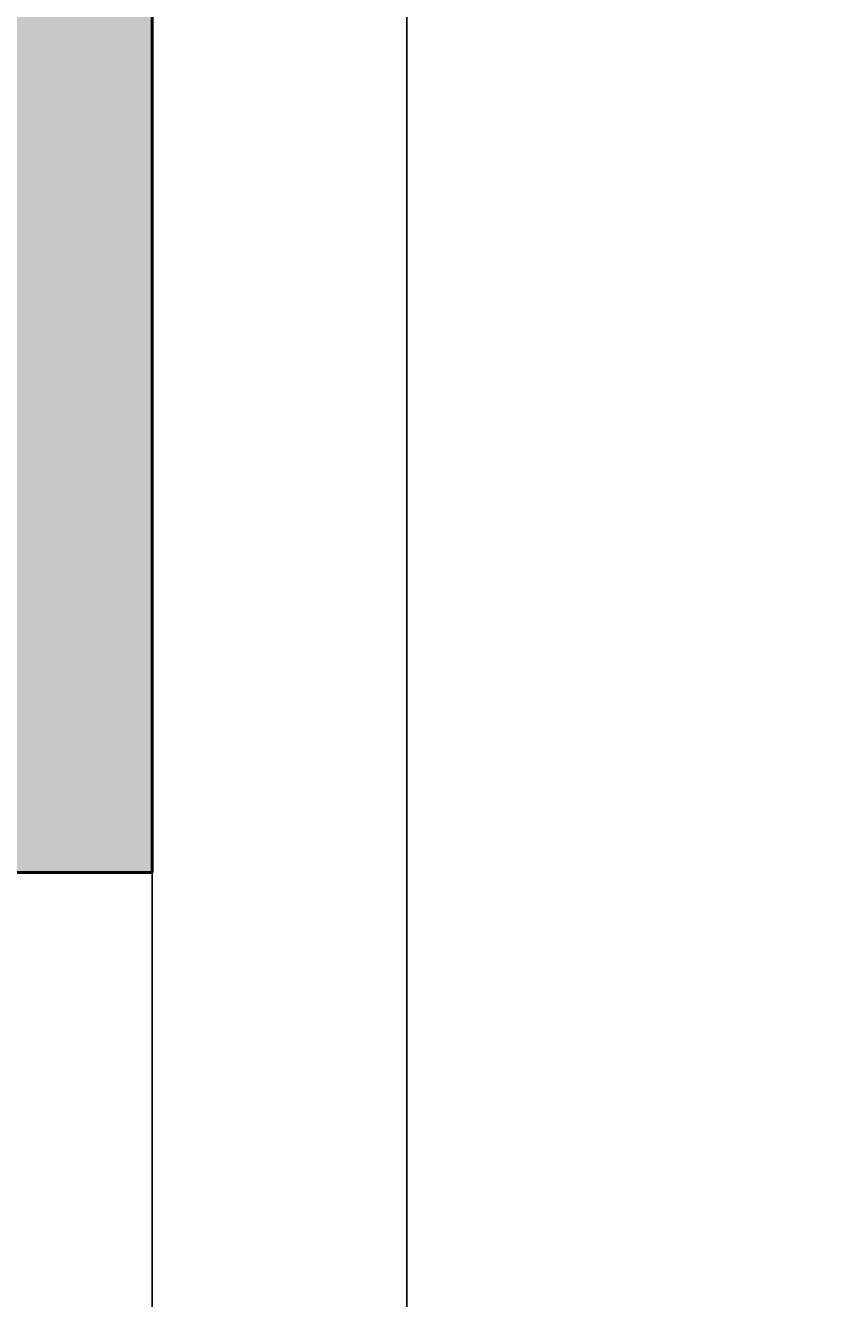
# Model space of a CAD drawing. Units: inches. Extents: x 2307 to 2544, y 2171 to 2540.
# Tile 34 of 52: x 2453 to 2472, y 2377 to 2407. Entities that reach past the tile are written whole.
import ezdxf

# ---------------------------------------------------------------- set-up
doc = ezdxf.new("R2010")
doc.units = ezdxf.units.IN
doc.layers.add('A-ANNO-DIMS', color=2, linetype='Continuous', lineweight=18)
doc.layers.add('A-WALL', color=7, linetype='Continuous', lineweight=50)
doc.layers.add('A-WALL-PATT', color=18, linetype='Continuous', lineweight=13, true_color=0x000000)
doc.styles.get("Standard").update_dxf_attribs({"font": 'arial.ttf'})
doc.dimstyles.get("Standard").update_dxf_attribs({"dimtxt": 0.18, "dimasz": 0.18, "dimexe": 0.18, "dimexo": 0.0625, "dimgap": 0.09, "dimtad": 0, "dimtih": 1, "dimtoh": 1, "dimdec": 4, "dimzin": 0, "dimdsep": 46, "dimtxsty": 'Standard', "dimcen": 0.09, "dimadec": 0, "dimazin": 0, "dimtfac": 1, "dimtdec": 4, "dimtofl": 0, "dimtmove": 0, "dimatfit": 3, "dimfxl": 1, "dimtolj": 1, "dimtzin": 0, "dimarcsym": 0})

# ---------------------------------------------------------------- blocks, each defined once
blk = doc.blocks.new('*D53')
at = {"layer": 'A-ANNO-DIMS', "color": 0, "lineweight": -2, "transparency": 16777216}
for p, q in [((2455.696, 2439.447), (2455.696, 2171.18)), ((2461.696, 2439.447), (2461.696, 2171.18)), ((2455.876, 2171.36), (2458.546, 2171.36)), ((2461.516, 2171.36), (2458.845, 2171.36))]:
    blk.add_line(p, q, dxfattribs=at)
at = {"layer": 'A-ANNO-DIMS', "color": 0, "transparency": 16777216}
for points in [[(2455.876, 2171.39), (2455.876, 2171.33), (2455.696, 2171.36)], [(2461.516, 2171.39), (2461.516, 2171.33), (2461.696, 2171.36)]]:
    blk.add_solid(points, dxfattribs=at)
at = {"layer": 'Defpoints', "color": 0, "transparency": 16777216}
for p in [(2455.696, 2439.51), (2461.696, 2439.51), (2461.696, 2171.36)]:
    blk.add_point(p, dxfattribs=at)
at = {"layer": 'A-ANNO-DIMS', "color": 0, "transparency": 16777216, "insert": (2458.696, 2171.36), "char_height": 0.18, "attachment_point": 5}
blk.add_mtext('\\A1;6', dxfattribs=at)
blk = doc.blocks.new('*D54')
at = {"layer": 'A-ANNO-DIMS', "color": 0, "lineweight": -2, "transparency": 16777216}
for p, q in [((2461.696, 2435.447), (2461.696, 2171.18)), ((2491.696, 2435.447), (2491.696, 2171.18)), ((2461.876, 2171.36), (2476.477, 2171.36)), ((2491.516, 2171.36), (2476.914, 2171.36))]:
    blk.add_line(p, q, dxfattribs=at)
at = {"layer": 'A-ANNO-DIMS', "color": 0, "transparency": 16777216}
for points in [[(2461.876, 2171.39), (2461.876, 2171.33), (2461.696, 2171.36)], [(2491.516, 2171.39), (2491.516, 2171.33), (2491.696, 2171.36)]]:
    blk.add_solid(points, dxfattribs=at)
at = {"layer": 'Defpoints', "color": 0, "transparency": 16777216}
for p in [(2461.696, 2435.51), (2491.696, 2435.51), (2491.696, 2171.36)]:
    blk.add_point(p, dxfattribs=at)
at = {"layer": 'A-ANNO-DIMS', "color": 0, "transparency": 16777216, "insert": (2476.696, 2171.36), "char_height": 0.18, "attachment_point": 5}
blk.add_mtext('\\A1;30', dxfattribs=at)
blk = doc.blocks.new('*D59')
at = {"layer": 'A-ANNO-DIMS', "color": 0, "lineweight": -2, "transparency": 16777216}
for p, q in [((2455.696, 2315.572), (2455.696, 2540.345)), ((2455.876, 2540.165), (2470.477, 2540.165)), ((2485.516, 2540.165), (2470.914, 2540.165)), ((2485.696, 2315.572), (2485.696, 2540.345))]:
    blk.add_line(p, q, dxfattribs=at)
at = {"layer": 'A-ANNO-DIMS', "color": 0, "transparency": 16777216}
for points in [[(2455.876, 2540.195), (2455.876, 2540.135), (2455.696, 2540.165)], [(2485.516, 2540.195), (2485.516, 2540.135), (2485.696, 2540.165)]]:
    blk.add_solid(points, dxfattribs=at)
at = {"layer": 'Defpoints', "color": 0, "transparency": 16777216}
for p in [(2455.696, 2540.165), (2455.696, 2315.51), (2485.696, 2315.51)]:
    blk.add_point(p, dxfattribs=at)
at = {"layer": 'A-ANNO-DIMS', "color": 0, "transparency": 16777216, "insert": (2470.696, 2540.165), "char_height": 0.18, "attachment_point": 5}
blk.add_mtext('\\A1;30', dxfattribs=at)

msp = doc.modelspace()

# ---------------------------------------------------------------- hatches: boundary and pattern name
at = {"layer": 'A-WALL-PATT'}
h = msp.add_hatch(color=256, dxfattribs=at)
h.dxf.hatch_style = 1
h.paths.add_polyline_path([(2433.6935, 2199.5096), (2415.6423, 2199.5096), (2415.6423, 2190.5096), (2433.7832, 2190.5096)], flags=17)
h.paths.add_polyline_path([(2367.6423, 2199.5096), (2335.6958, 2199.5096), (2335.6958, 2307.3983), (2326.6958, 2307.3983), (2326.6958, 2190.5096), (2367.6423, 2190.5096)])
h.paths.add_polyline_path([(2524.6958, 2520.5096), (2496.7832, 2520.5096), (2496.7832, 2515.5149), (2472.7832, 2515.5149), (2472.7832, 2520.5096), (2415.4028, 2520.5096), (2415.4028, 2511.5096), (2451.6958, 2511.5096), (2451.6958, 2439.5096), (2451.6958, 2391.5096), (2445.6958, 2391.5096), (2445.6958, 2387.5096), (2455.6958, 2387.5096), (2455.6958, 2435.5096), (2461.6958, 2435.5096), (2461.6958, 2439.5096), (2455.6958, 2439.5096), (2455.6958, 2511.5096), (2515.6958, 2511.5096), (2515.6958, 2439.5096), (2491.6958, 2439.5096), (2491.6958, 2435.5096), (2515.6958, 2435.5096), (2515.6958, 2319.5096), (2451.6958, 2319.5096), (2451.6958, 2281.5096), (2481.6958, 2281.5096), (2481.6958, 2225.5096), (2485.6958, 2225.5096), (2485.6958, 2285.5096), (2455.6958, 2285.5096), (2455.6958, 2315.5096), (2515.6958, 2315.5096), (2515.6958, 2199.5096), (2469.6952, 2199.5096), (2469.785, 2190.5096), (2524.6958, 2190.5096)])

# ---------------------------------------------------------------- linework, layer by layer
at = {"layer": 'A-WALL'}
for p, q in [((2455.6958, 2387.5096), (2455.6958, 2435.5096)), ((2455.6958, 2435.5096), (2455.6958, 2387.5096)), ((2445.6958, 2387.5096), (2455.6958, 2387.5096))]:
    msp.add_line(p, q, dxfattribs=at)

# ---------------------------------------------------------------- dimensions: what is measured, and where the dimension line sits
at = {"layer": 'A-ANNO-DIMS'}
for base, p1, p2, picture, middle in [((2455.6958, 2540.1649), (2485.6958, 2315.5096), (2455.6958, 2315.5096), '*D59', (2470.6958, 2540.1649)), ((2461.6958, 2171.3596), (2455.6958, 2439.5096), (2461.6958, 2439.5096), '*D53', (2458.6958, 2171.3596)), ((2491.6958, 2171.3596), (2461.6958, 2435.5096), (2491.6958, 2435.5096), '*D54', (2476.6958, 2171.3596))]:
    dim = msp.add_linear_dim(base=base, p1=p1, p2=p2, dimstyle='Standard', override={"dimdec": 0, "dimlfac": 1, "dimrnd": 0, "dimzin": 0, "dimdsep": 46, "dimlunit": 2}, dxfattribs=at)
    dim.commit()
    dim.dimension.update_dxf_attribs({"geometry": picture, "text_midpoint": middle})

doc.saveas('drawing.dxf')
